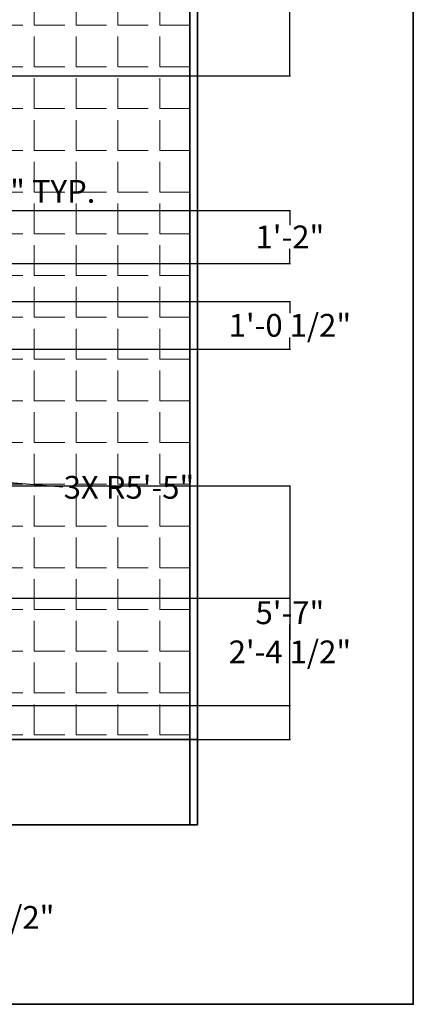
# Model space of a CAD drawing. Units: inches. Extents: x 1601 to 2080, y 5000 to 5589.
# Tile 6 of 11: x 1976 to 2080, y 5000 to 5259. Entities that reach past the tile are written whole.
import ezdxf

# ---------------------------------------------------------------- set-up
doc = ezdxf.new("R2010")
doc.units = ezdxf.units.IN
doc.header["$MEASUREMENT"] = 0
for name, color, linetype, lineweight in [('A-ANNO-DIMS', 2, 'Continuous', 18), ('A-ANNO-TTLB', 7, 'Continuous', 35), ('A-FLOR-PATT', 8, 'Continuous', 13), ('C-PROP', 7, 'Continuous', 35)]:
    doc.layers.add(name, color=color, linetype=linetype, lineweight=lineweight)
doc.styles.get("Standard").update_dxf_attribs({"font": 'arial.ttf'})
doc.dimstyles.get("Standard").update_dxf_attribs({"dimtxt": 6, "dimasz": 0.18, "dimexe": 0.18, "dimexo": 0.0625, "dimgap": 0.09, "dimtad": 0, "dimtih": 1, "dimtoh": 1, "dimdec": 1, "dimzin": 0, "dimdsep": 46, "dimlunit": 3, "dimtxsty": 'Standard', "dimcen": 0.09, "dimadec": 0, "dimazin": 0, "dimtfac": 1, "dimtdec": 1, "dimtofl": 0, "dimtmove": 0, "dimatfit": 3, "dimfxl": 1, "dimtolj": 1, "dimtzin": 0, "dimarcsym": 0})

# ---------------------------------------------------------------- blocks, each defined once
blk = doc.blocks.new('*D33')
at = {"layer": 'A-ANNO-DIMS', "color": 0, "lineweight": -2, "transparency": 16777216}
for p, q in [((1962.97, 5219.2), (1964.59, 5219.2)), ((1964.41, 5219.02), (1964.41, 5217.35)), ((1964.41, 5209.38), (1964.41, 5211.04)), ((1962.97, 5209.2), (1964.59, 5209.2))]:
    blk.add_line(p, q, dxfattribs=at)
at = {"layer": 'A-ANNO-DIMS', "color": 0, "transparency": 16777216}
for points in [[(1964.38, 5219.02), (1964.44, 5219.02), (1964.41, 5219.2)], [(1964.38, 5209.38), (1964.44, 5209.38), (1964.41, 5209.2)]]:
    blk.add_solid(points, dxfattribs=at)
at = {"layer": 'Defpoints', "color": 0, "transparency": 16777216}
for p in [(1962.91, 5219.2), (1962.91, 5209.2), (1964.41, 5209.2)]:
    blk.add_point(p, dxfattribs=at)
at = {"layer": 'A-ANNO-DIMS', "color": 0, "transparency": 16777216, "insert": (1964.41, 5214.2), "char_height": 6, "attachment_point": 5}
blk.add_mtext('\\A1;VENT 0\'-10" TYP.', dxfattribs=at)
blk = doc.blocks.new('*D44')
at = {"layer": 'A-ANNO-DIMS', "color": 0, "lineweight": -2, "transparency": 16777216}
for p, q in [((1929.65, 5106.89), (1929.65, 5022.68)), ((1953.91, 5078.63), (1953.91, 5022.68)), ((1929.83, 5022.86), (1953.73, 5022.86)), ((1953.91, 5022.86), (1954.09, 5022.86))]:
    blk.add_line(p, q, dxfattribs=at)
at = {"layer": 'A-ANNO-DIMS', "color": 0, "transparency": 16777216}
for points in [[(1929.83, 5022.89), (1929.83, 5022.83), (1929.65, 5022.86)], [(1953.73, 5022.89), (1953.73, 5022.83), (1953.91, 5022.86)]]:
    blk.add_solid(points, dxfattribs=at)
at = {"layer": 'Defpoints', "color": 0, "transparency": 16777216}
for p in [(1929.65, 5106.95), (1953.91, 5078.7), (1953.91, 5022.86)]:
    blk.add_point(p, dxfattribs=at)
at = {"layer": 'A-ANNO-DIMS', "color": 0, "transparency": 16777216, "insert": (1969.19, 5022.86), "char_height": 6, "attachment_point": 5}
blk.add_mtext('\\A1;2\'-0 1/2"', dxfattribs=at)
blk = doc.blocks.new('*D45')
at = {"layer": 'A-ANNO-DIMS', "color": 0, "lineweight": -2, "transparency": 16777216}
for p, q in [((1833.97, 5106.95), (2047.44, 5106.95)), ((2047.26, 5106.77), (2047.26, 5096.02)), ((2047.26, 5078.88), (2047.26, 5089.63)), ((1829.47, 5078.7), (2047.44, 5078.7))]:
    blk.add_line(p, q, dxfattribs=at)
at = {"layer": 'A-ANNO-DIMS', "color": 0, "transparency": 16777216}
for points in [[(2047.23, 5106.77), (2047.29, 5106.77), (2047.26, 5106.95)], [(2047.23, 5078.88), (2047.29, 5078.88), (2047.26, 5078.7)]]:
    blk.add_solid(points, dxfattribs=at)
at = {"layer": 'Defpoints', "color": 0, "transparency": 16777216}
for p in [(1833.91, 5106.95), (2047.26, 5106.95), (1829.41, 5078.7)]:
    blk.add_point(p, dxfattribs=at)
at = {"layer": 'A-ANNO-DIMS', "color": 0, "transparency": 16777216, "insert": (2047.26, 5092.83), "char_height": 6, "attachment_point": 5}
blk.add_mtext('\\A1;2\'-4 1/2"', dxfattribs=at)
blk = doc.blocks.new('*D50')
at = {"layer": 'A-ANNO-DIMS', "color": 0, "lineweight": -2, "transparency": 16777216}
for p, q in [((1962.97, 5136.6), (2047.44, 5136.6)), ((2047.26, 5136.42), (2047.26, 5106.29)), ((2047.26, 5069.88), (2047.26, 5100.01)), ((1962.97, 5069.7), (2047.44, 5069.7))]:
    blk.add_line(p, q, dxfattribs=at)
at = {"layer": 'A-ANNO-DIMS', "color": 0, "transparency": 16777216}
for points in [[(2047.23, 5136.42), (2047.29, 5136.42), (2047.26, 5136.6)], [(2047.23, 5069.88), (2047.29, 5069.88), (2047.26, 5069.7)]]:
    blk.add_solid(points, dxfattribs=at)
at = {"layer": 'Defpoints', "color": 0, "transparency": 16777216}
for p in [(1962.91, 5136.6), (2047.26, 5136.6), (1962.91, 5069.7)]:
    blk.add_point(p, dxfattribs=at)
at = {"layer": 'A-ANNO-DIMS', "color": 0, "transparency": 16777216, "insert": (2047.26, 5103.15), "char_height": 6, "attachment_point": 5}
blk.add_mtext('\\A1;5\'-7"', dxfattribs=at)
blk = doc.blocks.new('*D54')
at = {"layer": 'A-ANNO-DIMS', "color": 0, "lineweight": -2, "transparency": 16777216}
for p, q in [((1962.97, 5209.2), (2047.44, 5209.2)), ((2047.26, 5209.02), (2047.26, 5205.3)), ((2047.26, 5195.38), (2047.26, 5199.09)), ((1962.97, 5195.2), (2047.44, 5195.2))]:
    blk.add_line(p, q, dxfattribs=at)
at = {"layer": 'A-ANNO-DIMS', "color": 0, "transparency": 16777216}
for points in [[(2047.23, 5209.02), (2047.29, 5209.02), (2047.26, 5209.2)], [(2047.23, 5195.38), (2047.29, 5195.38), (2047.26, 5195.2)]]:
    blk.add_solid(points, dxfattribs=at)
at = {"layer": 'Defpoints', "color": 0, "transparency": 16777216}
for p in [(1962.91, 5209.2), (2047.26, 5209.2), (1962.91, 5195.2)]:
    blk.add_point(p, dxfattribs=at)
at = {"layer": 'A-ANNO-DIMS', "color": 0, "transparency": 16777216, "insert": (2047.26, 5202.2), "char_height": 6, "attachment_point": 5}
blk.add_mtext('\\A1;1\'-2"', dxfattribs=at)
blk = doc.blocks.new('*D55')
at = {"layer": 'A-ANNO-DIMS', "color": 0, "lineweight": -2, "transparency": 16777216}
for p, q in [((1962.97, 5185.2), (2047.44, 5185.2)), ((2047.26, 5185.02), (2047.26, 5182.09)), ((2047.26, 5172.78), (2047.26, 5175.71)), ((1962.97, 5172.6), (2047.44, 5172.6))]:
    blk.add_line(p, q, dxfattribs=at)
at = {"layer": 'A-ANNO-DIMS', "color": 0, "transparency": 16777216}
for points in [[(2047.23, 5185.02), (2047.29, 5185.02), (2047.26, 5185.2)], [(2047.23, 5172.78), (2047.29, 5172.78), (2047.26, 5172.6)]]:
    blk.add_solid(points, dxfattribs=at)
at = {"layer": 'Defpoints', "color": 0, "transparency": 16777216}
for p in [(1962.91, 5185.2), (2047.26, 5185.2), (1962.91, 5172.6)]:
    blk.add_point(p, dxfattribs=at)
at = {"layer": 'A-ANNO-DIMS', "color": 0, "transparency": 16777216, "insert": (2047.26, 5178.9), "char_height": 6, "attachment_point": 5}
blk.add_mtext('\\A1;1\'-0 1/2"', dxfattribs=at)
blk = doc.blocks.new('*D56')
at = {"layer": 'A-ANNO-DIMS', "color": 0, "lineweight": -2, "transparency": 16777216}
for p, q in [((1833.97, 5300.2), (2047.44, 5300.2)), ((2047.26, 5300.02), (2047.26, 5275.61)), ((2047.26, 5244.82), (2047.26, 5269.23)), ((1833.97, 5244.64), (2047.44, 5244.64))]:
    blk.add_line(p, q, dxfattribs=at)
at = {"layer": 'A-ANNO-DIMS', "color": 0, "transparency": 16777216}
for points in [[(2047.23, 5300.02), (2047.29, 5300.02), (2047.26, 5300.2)], [(2047.23, 5244.82), (2047.29, 5244.82), (2047.26, 5244.64)]]:
    blk.add_solid(points, dxfattribs=at)
at = {"layer": 'Defpoints', "color": 0, "transparency": 16777216}
for p in [(1833.91, 5300.2), (2047.26, 5300.2), (1833.91, 5244.64)]:
    blk.add_point(p, dxfattribs=at)
at = {"layer": 'A-ANNO-DIMS', "color": 0, "transparency": 16777216, "insert": (2047.26, 5272.42), "char_height": 6, "attachment_point": 5}
blk.add_mtext('\\A1;4\'-7 1/2"', dxfattribs=at)
blk = doc.blocks.new('*D63')
at = {"layer": 'A-ANNO-DIMS', "color": 0, "lineweight": -2, "transparency": 16777216}
for p, q in [((1883.68, 5145.05), (1883.86, 5145.05)), ((1883.77, 5144.96), (1883.77, 5145.14)), ((1987.53, 5136.21), (1948.8, 5139.51))]:
    blk.add_line(p, q, dxfattribs=at)
at = {"layer": 'A-ANNO-DIMS', "color": 0, "transparency": 16777216}
blk.add_solid([(1948.8, 5139.54), (1948.8, 5139.48), (1948.62, 5139.53)], dxfattribs=at)
at = {"layer": 'Defpoints', "color": 0, "transparency": 16777216}
for p in [(1883.77, 5145.05), (1948.62, 5139.53)]:
    blk.add_point(p, dxfattribs=at)
at = {"layer": 'A-ANNO-DIMS', "color": 0, "transparency": 16777216, "insert": (2004.91, 5136.21), "char_height": 6, "attachment_point": 5}
blk.add_mtext('\\A1;3X R5\'-5"', dxfattribs=at)

msp = doc.modelspace()

# ---------------------------------------------------------------- hatches: boundary and pattern name
at = {"layer": 'A-FLOR-PATT'}
h = msp.add_hatch(dxfattribs=at)
h.set_pattern_fill('ANGLE', color=256, scale=40)
h.set_pattern_definition([(0, (0, 0), (0, 11), [8, -3]), (90, (0, 0), (-11, 7e-16), [8, -3])])
h.paths.add_polyline_path([(2022.91, 5509.2), (1941.91, 5509.2), (1911.91, 5509.2), (1864.41, 5509.2), (1864.41, 5489.7), (1868.54, 5489.7, -0.022155), (1868.52, 5490.01, -1), (1875.53, 5490.01, -0.956651), (1868.54, 5489.7), (1864.41, 5489.7), (1864.41, 5470.2), (1794.41, 5470.2), (1794.41, 5431.2), (1811.95, 5431.2), (1911.91, 5431.2), (1941.91, 5431.2), (1942.91, 5431.2), (1945.91, 5431.2), (1948.91, 5431.2), (1962.91, 5431.2), (1962.91, 5415.29), (1962.91, 5385.29), (1962.91, 5384.29), (1962.91, 5381.29), (1962.91, 5333.29), (1962.91, 5069.7), (2022.91, 5069.7)])
h.paths.add_polyline_path([(2000.28, 5267.55), (2000.28, 5367.64), (1987.91, 5367.64), (1987.91, 5267.55)], flags=24)
h.paths.add_polyline_path([(1879.42, 5455.52), (1969.04, 5455.52), (1969.04, 5467.88), (1879.42, 5467.88)], flags=24)

# ---------------------------------------------------------------- linework, layer by layer
at = {"layer": 'A-ANNO-TTLB'}
msp.add_lwpolyline([(1600.55, 5589.45), (2079.72, 5589.45), (2079.72, 4999.95), (1600.55, 4999.95)], close=True, dxfattribs=at)
at = {"layer": 'C-PROP'}
for p, q in [((2020.91, 5509.2), (2020.91, 5047.21)), ((2022.91, 5509.2), (2022.91, 5047.21)), ((2022.91, 5069.7), (1962.91, 5069.7)), ((1664.41, 5047.21), (2022.91, 5047.21))]:
    msp.add_line(p, q, dxfattribs=at)

# ---------------------------------------------------------------- dimensions: what is measured, and where the dimension line sits
at = {"layer": 'A-ANNO-DIMS'}
for base, p1, p2, picture, middle in [((2047.26, 5300.2), (1833.91, 5244.64), (1833.91, 5300.2), '*D56', (2047.26, 5272.42)), ((2047.26, 5209.2), (1962.91, 5195.2), (1962.91, 5209.2), '*D54', (2047.26, 5202.2)), ((2047.26, 5185.2), (1962.91, 5172.6), (1962.91, 5185.2), '*D55', (2047.26, 5178.9)), ((2047.26, 5136.6), (1962.91, 5069.7), (1962.91, 5136.6), '*D50', (2047.26, 5103.15)), ((2047.2582, 5106.9548), (1829.4082, 5078.6964), (1833.9082, 5106.9548), '*D45', (2047.2582, 5092.8256))]:
    dim = msp.add_linear_dim(base=base, p1=p1, p2=p2, angle=90, dimstyle='Standard', override={"dimdec": 1, "dimlfac": 1, "dimrnd": 0, "dimzin": 1, "dimdsep": 46, "dimlunit": 4, "dimfrac": 2}, dxfattribs=at)
    dim.commit()
    dim.dimension.update_dxf_attribs({"geometry": picture, "text_midpoint": middle})
dim = msp.add_linear_dim(base=(1964.41, 5209.2), p1=(1962.91, 5219.2), p2=(1962.91, 5209.2), angle=270, text='VENT <> TYP.', dimstyle='Standard', override={"dimdec": 1, "dimlfac": 1, "dimrnd": 0, "dimzin": 1, "dimdsep": 46, "dimlunit": 4, "dimfrac": 2}, dxfattribs=at)
dim.commit()
dim.dimension.update_dxf_attribs({"geometry": '*D33', "text_midpoint": (1964.41, 5214.2)})
dim = msp.add_radius_dim(center=(1883.77, 5145.05), mpoint=(1948.62, 5139.53), text='3X <>', dimstyle='Standard', override={"dimdec": 1, "dimlfac": 1, "dimrnd": 0, "dimzin": 1, "dimdsep": 46, "dimlunit": 4, "dimfrac": 2}, dxfattribs=at)
dim.commit()
dim.dimension.update_dxf_attribs({"geometry": '*D63', "text_midpoint": (1987.53, 5136.21), "dimtype": 164})
dim = msp.add_linear_dim(base=(1953.91, 5022.86), p1=(1929.65, 5106.95), p2=(1953.91, 5078.7), dimstyle='Standard', override={"dimdec": 1, "dimlfac": 1, "dimrnd": 0, "dimzin": 1, "dimdsep": 46, "dimlunit": 4, "dimfrac": 2}, dxfattribs=at)
dim.commit()
dim.dimension.update_dxf_attribs({"geometry": '*D44', "text_midpoint": (1969.19, 5022.86)})

doc.saveas('drawing.dxf')
